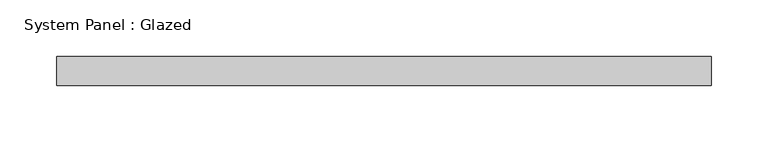
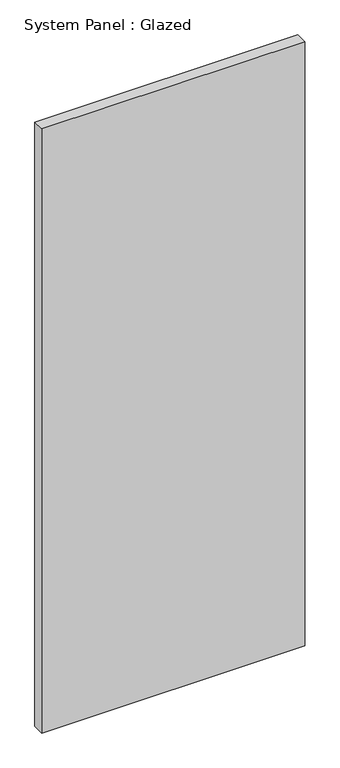
"""IFC4 building model written with IfcOpenShell, lengths in millimetres: plate geometry, System Panel : Glazed."""

from ifc_helpers import new_model, si_unit, origin, origin_with_axes, place, context, project, spatial, polyline, outline, extrude, source, transform, mapped, element, save


def system_panel_glazed_a6da17b0(model_context):
    return source(origin(), model_context, "Body", "SweptSolid", [
        extrude(outline(polyline([(287.133278, 19.05), (-287.133278, 19.05), (-287.133278, 44.45), (287.133278, 44.45), (287.133278, 19.05)])), origin_with_axes(), (0.0, 0.0, 1.0), 1394.9137173),
    ])


if __name__ == "__main__":
    model = new_model("IFC4")
    model_context = context("Model", 3, world=origin())
    ifc_project = project(units=[si_unit("LENGTHUNIT", "METRE", prefix="MILLI")], contexts=[model_context])
    site = spatial("IfcSite", under=ifc_project)
    building = spatial("IfcBuilding", under=site)
    placement = place(None, origin())
    system_panel_glazed_shape = system_panel_glazed_a6da17b0(model_context)
    element("IfcPlate", 1, ObjectType="System Panel : Glazed", at=placement, inside=building, context=model_context, shape_type="MappedRepresentation", body=[
        mapped(system_panel_glazed_shape, transform((0.0, 0.0, 0.0), x_axis=(1.0, 0.0, 0.0), y_axis=(0.0, 1.0, 0.0), z_axis=(0.0, 0.0, 1.0))),
    ])
    save(model, "model.ifc")

# Revit data of these elements
# Type "System Panel : Glazed"
#   Construction Type Id = "GSP4R"
#   Analytic Construction = "1/8 in Pilkington single glazing"
#   Visual Light Transmittance = 0.9
#   Solar Heat Gain Coefficient = 0.86
#   Heat Transfer Coefficient (U) = 1.18115 BTU/(h·ft²·°F)
#   Define Thermal Properties by = 1
# Element 1 (IfcPlate, "System Panel : Glazed")
#   Materials on its faces: "Glass"
# Materials
#   "Glass": class "Glass", colour RGB 0 128 192, transparency 0.75, Description = "Soda Lime Glass", Cost = 0
